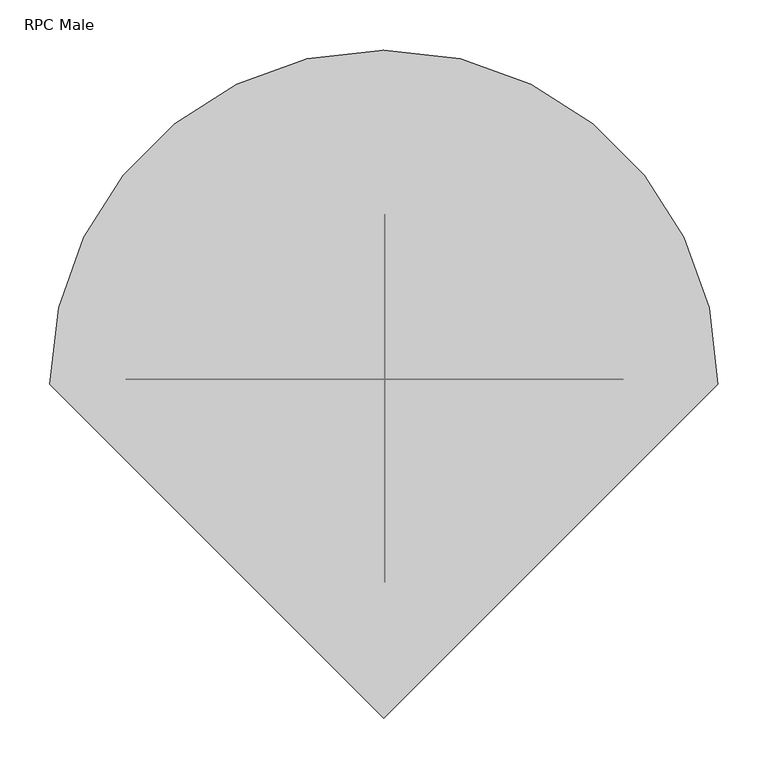
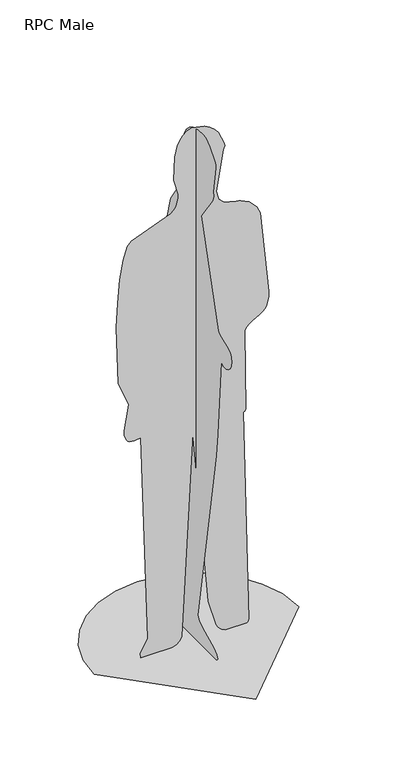
"""IFC4 building model written with IfcOpenShell, lengths in millimetres: proxy geometry, RPC Male."""

from ifc_helpers import new_model, si_unit, origin, place, context, project, spatial, triangles, source, transform, mapped, element, save


def rpc_male_28878092(model_context):
    return source(origin(), model_context, "Body", "Tessellation", [
        triangles([(180.7519758, 4.45e-05, 5.61e-05), (184.2427693, 8.8e-06, 2.7953145), (186.1721755, -1.66e-05, 5.8375002), (186.8316374, -3.35e-05, 9.127569), (168.2846227, -8.5e-06, 733.0652109), (173.8813015, -8.5e-06, 735.2240908), (177.6698602, -8.1e-06, 740.93319), (174.1985423, 8.1e-06, 1013.6682867), (179.591309, 8.8e-06, 1024.1651751), (188.0395216, 9.6e-06, 1032.7759867), (198.5267085, 9.9e-06, 1040.1126028), (210.0363257, 1.03e-05, 1046.7864687), (221.5520472, 1.07e-05, 1053.4092476), (232.0572199, 1.1e-05, 1060.5929661), (240.5353907, 1.14e-05, 1068.9488514), (245.9518842, 1.21e-05, 1078.9880642), (249.7386988, 1.29e-05, 1091.9821838), (252.1552483, 1.4e-05, 1106.9298906), (253.4607645, 1.47e-05, 1122.8295742), (224.2188539, 3.16e-05, 1405.054644), (213.7949444, 3.31e-05, 1430.2019463), (189.1319694, 3.46e-05, 1456.0842327), (160.624934, 3.53e-05, 1468.8737137), (131.9229886, 3.57e-05, 1475.6378357), (106.6752928, 3.64e-05, 1483.4436092), (88.5310242, 3.71e-05, 1499.3593529), (81.1392697, 3.9e-05, 1530.4516411), (102.942045, 4.71e-05, 1666.4696468), (107.9472446, 4.78e-05, 1679.2650867), (108.1474504, 4.82e-05, 1680.5741638), (107.984815, 4.82e-05, 1682.7587688), (107.5268306, 4.82e-05, 1685.5190655), (106.840944, 4.86e-05, 1688.5553627), (86.6409052, 5.11e-05, 1733.0902897), (74.2774293, 5.19e-05, 1747.7183212), (59.5121605, 5.26e-05, 1759.6594528), (42.363121, 5.33e-05, 1768.7777916), (0.9855255, 5.37e-05, 1777.9990311), (-15.8808757, 5.33e-05, 1772.5528519), (-29.1619555, 5.26e-05, 1761.5639877), (-39.2640369, 5.19e-05, 1747.0962662), (-46.5934632, 5.08e-05, 1731.2140961), (-56.009163, 4.89e-05, 1695.7207684), (-59.1639487, 4.41e-05, 1618.2087845), (-44.4858339, 4.12e-05, 1564.7278919), (-44.3096682, 4.05e-05, 1551.1862766), (-46.5532813, 3.94e-05, 1537.9279289), (-51.2886345, 3.86e-05, 1525.4359589), (-58.5876575, 3.83e-05, 1514.1926044), (-68.5223164, 3.75e-05, 1504.6808304), (-198.4030241, 3.46e-05, 1454.5808361), (-210.7095586, 3.38e-05, 1440.8296406), (-224.9005892, 3.13e-05, 1397.8447643), (-235.5369131, 2.72e-05, 1333.6069702), (-242.7580384, 2.28e-05, 1256.1532677), (-246.7032373, 1.77e-05, 1173.5211021), (-240.2781571, 5.9e-06, 974.9290089), (-206.081389, 1.1e-06, 891.6222479), (-221.1961823, -4e-06, 805.6633232), (-220.4650678, -5.1e-06, 788.6200321), (-214.9948893, -6.3e-06, 771.8045614), (-210.3552016, -6.6e-06, 765.7300776), (-204.1668257, -6.6e-06, 762.0919275), (-196.8959759, -7e-06, 760.3982082), (-189.0090118, -7e-06, 760.1573799), (-180.9721295, -7e-06, 760.8774668), (-173.2515615, -6.6e-06, 762.0669291), (-166.3135766, -6.6e-06, 763.2339363), (-144.8011179, -4.49e-05, 59.4752896), (-168.6275342, -4.74e-05, 15.3365843), (-166.1985945, 4.45e-05, 5.61e-05), (-66.1332089, 4.45e-05, 5.61e-05), (-49.8425018, 1.03e-05, 3.9765591), (-39.0246256, -1.36e-05, 14.0353), (-32.5983009, -2.91e-05, 28.3297116), (2.7441046, -9.2e-06, 720.0458748), (54.0725034, -1.03e-05, 117.9433278), (81.3720135, 2.13e-05, 28.0047427), (85.5237041, 2.69e-05, 19.9172686), (91.2433859, 3.27e-05, 12.5691172), (99.2451413, 3.86e-05, 5.9378887), (110.2431982, 4.45e-05, 5.61e-05), (13.8237406, 127.6718764, 9.9621145), (13.8237974, 127.2617633, 182.0842528), (13.8237815, 135.2635732, 744.8695776), (13.8237815, 136.4149928, 748.3460369), (13.8237815, 139.3954704, 752.5736132), (13.8237815, 143.4944026, 757.5058702), (13.8237815, 148.0010861, 763.0962994), (13.8237815, 152.2049901, 769.2983917), (13.8237792, 155.3953659, 776.0656385), (13.8237792, 156.8616281, 783.3516764), (13.8237622, 165.9465024, 1358.6137287), (13.8237599, 143.2743216, 1442.0927902), (13.8237576, 71.1145501, 1552.8585583), (13.8237576, 64.3401725, 1580.5206779), (13.8237542, 73.5344014, 1684.7952724), (13.8237531, 67.2131212, 1712.2161278), (13.8237531, 55.241223, 1734.9070393), (13.8237531, 37.9260212, 1752.7537697), (13.8237531, 15.5748771, 1765.6426632), (13.8237531, -11.5049084, 1773.4593372), (13.8237531, -43.0059914, 1776.090136), (13.8237531, -55.0860226, 1772.9164925), (13.8237542, -79.7038559, 1756.3218658), (13.8237554, -107.4896145, 1722.3477768), (13.8237554, -111.5711695, 1713.01012), (13.8237554, -112.2229284, 1702.3019073), (13.8237588, -99.0832235, 1611.9284992), (13.8237588, -100.6007272, 1597.8206394), (13.8237599, -96.755177, 1579.0656796), (13.8237622, -31.1784566, 1488.4592915), (13.8237735, -125.7984261, 1146.7472277), (13.8237735, -134.1993577, 1137.675107), (13.8237747, -184.2799037, 1119.3925747), (13.8237747, -194.4649651, 1111.9394686), (13.8237747, -201.1343255, 1100.3801451), (13.8237769, -203.5508567, 1084.2058416), (13.8237769, -200.9674025, 1068.9640394), (13.8237769, -194.2820729, 1055.8707253), (13.8237769, -184.3928146, 1046.1415226), (13.8237769, -172.1978105, 1040.992709), (13.8237769, -158.595007, 1041.6399078), (13.8237769, -144.48246, 1049.299106), (13.8237838, -123.0429529, 785.7648285), (13.823786, -116.906318, 707.2429499), (13.8237928, -10.2023683, 90.6853168), (13.823794, -17.983895, 76.1481908), (13.8237951, -35.4714404, 63.806743), (13.8238042, -104.5965316, 31.8661463), (13.8238053, -119.3344402, 20.2173661), (13.8238076, -122.9915025, 6.7192091), (13.8238042, -122.0607091, 4.3674998), (13.8237894, -120.3451706, 2.3141478), (13.8237724, -119.1853577, 1.4285653), (13.8237474, -117.8199432, 0.6534771), (13.8237099, -116.2458387, 5.61e-05), (13.8237077, 124.501612, 0.0), (348.4734607, -4.7230039, 0.0001684), (339.5987117, 72.1961519, 0.0001684), (314.3237646, 142.8340959, 5.61e-05), (274.6722241, 205.1669827, 5.61e-05), (222.6681673, 257.171094, 5.61e-05), (160.3352533, 296.8225073, 5.61e-05), (89.6973139, 322.097527, 5.61e-05), (12.7781649, 330.972276, 5.61e-05), (-64.1409886, 322.0975634, 5.61e-05), (-134.7789371, 296.8225618, 5.61e-05), (-197.1118239, 257.1710577, 5.61e-05), (-249.1159897, 205.1670008, 5.61e-05), (-288.7673667, 142.8340595, 5.61e-05), (-314.0423864, 72.1960974, 0.0001684), (-322.9171354, -4.7230331, 0.0001684), (12.7782239, -340.4182474, 0.0001684)], [[70, 71, 72], [69, 70, 72], [69, 72, 73], [69, 73, 74], [69, 74, 75], [69, 75, 76], [68, 69, 76], [82, 1, 2], [82, 2, 3], [82, 3, 4], [81, 82, 4], [80, 81, 4], [79, 80, 4], [78, 79, 4], [77, 78, 4], [77, 4, 5], [76, 77, 5], [5, 6, 7], [76, 5, 7], [76, 7, 8], [68, 76, 8], [67, 68, 8], [66, 67, 8], [65, 66, 8], [64, 65, 8], [63, 64, 8], [62, 63, 8], [61, 62, 8], [60, 61, 8], [59, 60, 8], [58, 59, 8], [57, 58, 8], [56, 57, 8], [56, 8, 9], [55, 56, 9], [55, 9, 10], [54, 55, 10], [54, 10, 11], [53, 54, 11], [53, 11, 12], [52, 53, 12], [51, 52, 12], [50, 51, 12], [50, 12, 13], [50, 13, 14], [50, 14, 15], [50, 15, 16], [50, 16, 17], [50, 17, 18], [50, 18, 19], [50, 19, 20], [50, 20, 21], [50, 21, 22], [50, 22, 23], [50, 23, 24], [50, 24, 25], [50, 25, 26], [49, 50, 26], [48, 49, 26], [48, 26, 27], [47, 48, 27], [46, 47, 27], [45, 46, 27], [44, 45, 27], [44, 27, 28], [43, 44, 28], [42, 43, 28], [42, 28, 29], [42, 29, 30], [42, 30, 31], [42, 31, 32], [42, 32, 33], [42, 33, 34], [42, 34, 35], [42, 35, 36], [42, 36, 37], [41, 42, 37], [40, 41, 37], [40, 37, 38], [40, 38, 39], [137, 138, 83], [137, 83, 84], [136, 137, 84], [135, 136, 84], [130, 131, 132], [130, 132, 133], [130, 133, 134], [130, 134, 135], [122, 123, 124], [121, 122, 124], [120, 121, 124], [119, 120, 124], [118, 119, 124], [117, 118, 124], [116, 117, 124], [115, 116, 124], [114, 115, 124], [113, 114, 124], [106, 107, 108], [105, 106, 108], [104, 105, 108], [103, 104, 108], [102, 103, 108], [101, 102, 108], [100, 101, 108], [99, 100, 108], [98, 99, 108], [97, 98, 108], [97, 108, 109], [97, 109, 110], [97, 110, 111], [96, 97, 111], [95, 96, 111], [95, 111, 112], [94, 95, 112], [93, 94, 112], [93, 112, 113], [92, 93, 113], [92, 113, 124], [92, 124, 125], [91, 92, 125], [90, 91, 125], [89, 90, 125], [88, 89, 125], [87, 88, 125], [86, 87, 125], [86, 125, 126], [85, 86, 126], [85, 126, 127], [84, 85, 127], [84, 127, 128], [135, 84, 128], [135, 128, 129], [130, 135, 129], [153, 154, 139], [152, 153, 139], [152, 139, 140], [151, 152, 140], [151, 140, 141], [151, 141, 142], [150, 151, 142], [149, 150, 142], [149, 142, 143], [149, 143, 144], [149, 144, 145], [149, 145, 146], [149, 146, 147], [149, 147, 148]], closed=False),
    ])


if __name__ == "__main__":
    model = new_model("IFC4")
    model_context = context("Model", 3, world=origin())
    ifc_project = project(units=[si_unit("LENGTHUNIT", "METRE", prefix="MILLI")], contexts=[model_context])
    site = spatial("IfcSite", under=ifc_project)
    building = spatial("IfcBuilding", under=site)
    placement = place(None, origin())
    rpc_male_shape = rpc_male_28878092(model_context)
    element("IfcBuildingElementProxy", 1, Name="RPC Male", ObjectType="RPC Male", at=placement, inside=building, context=model_context, shape_type="MappedRepresentation", body=[
        mapped(rpc_male_shape, transform((0.0, 0.0, 0.0), x_axis=(1.0, 0.0, 0.0), y_axis=(0.0, 1.0, 0.0), z_axis=(0.0, 0.0, 1.0))),
    ])
    save(model, "model.ifc")

# Revit data of these elements
# Type "RPC Male"
#   built-in parameter 1005195 = "RPC-8-G1AE-S4G0-CKUK-A"
#   Height = 0
